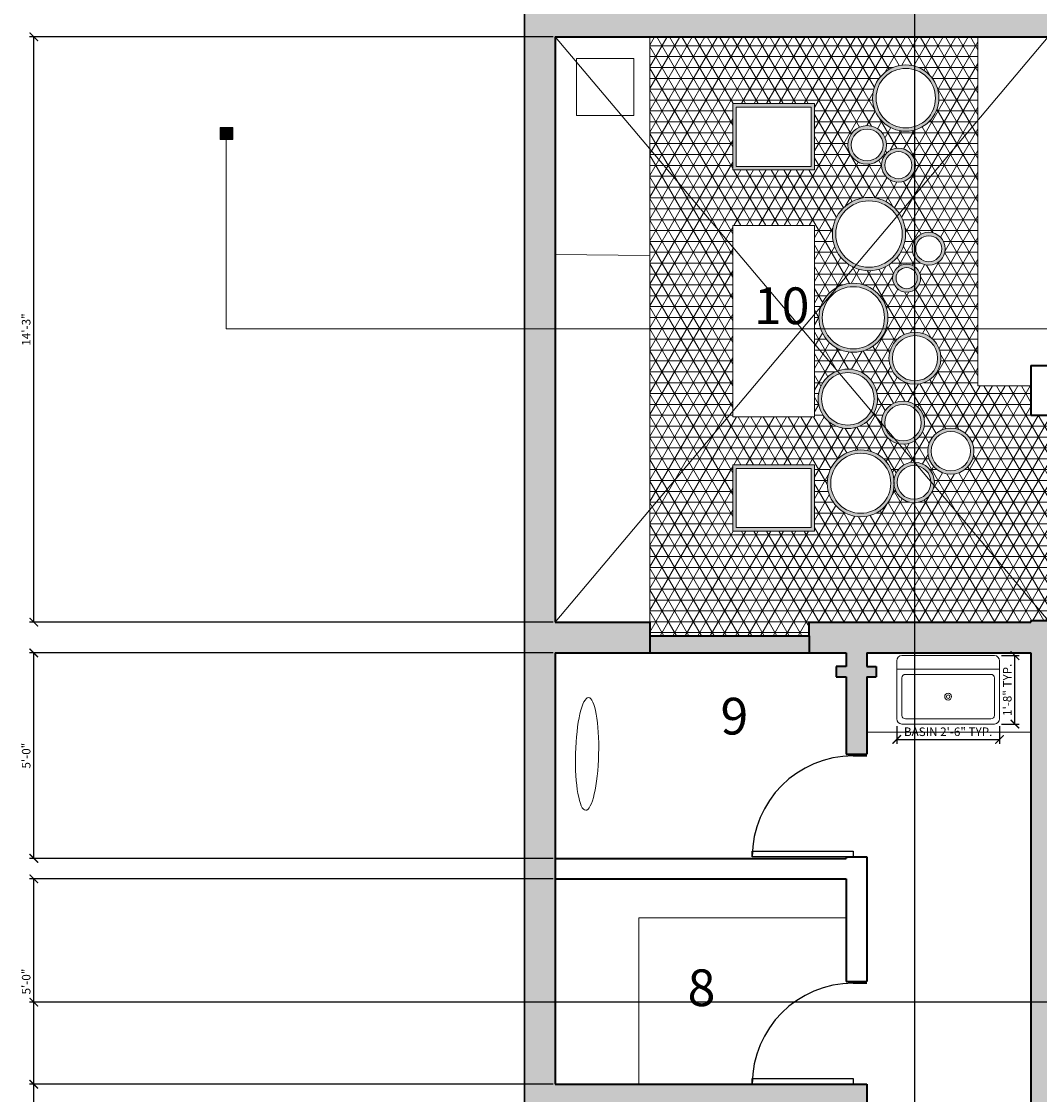
# Model space of a CAD drawing. Units: inches. Extents: x 3122 to 5933, y 1474 to 2995.
# Tile 5 of 12: x 4918 to 5215, y 2326 to 2639. Entities that reach past the tile are written whole.
import ezdxf

# ---------------------------------------------------------------- set-up
doc = ezdxf.new("R2010")
doc.units = ezdxf.units.IN
for name, color, linetype, lineweight in [('A-ANNO-DIMS', 2, 'Continuous', 18), ('A-ANNO-SYMB', 6, 'Continuous', 18), ('A-AREA-IDEN', 7, 'Continuous', 20), ('A-DOOR', 4, 'Continuous', 25), ('A-FLOR-CASE', 8, 'Continuous', 18), ('A-FLOR-FIXT', 9, 'Continuous', 18), ('A-FLOR-OPEN', 8, 'Continuous', 13), ('A-WALL', 7, 'Continuous', 35), ('A-WALL-PATT', 7, 'Continuous', 13), ('C-PROP', 7, 'Continuous', 25), ('L-PLNT', 3, 'Continuous', 18), ('L-PLNT-PATT', 94, 'Continuous', 13)]:
    doc.layers.add(name, color=color, linetype=linetype, lineweight=lineweight)
doc.styles.get("Standard").update_dxf_attribs({"font": 'arial.ttf'})
doc.dimstyles.new('ISO-25', dxfattribs={"dimtxt": 2.5, "dimasz": 2.5, "dimexe": 1.25, "dimexo": 0.625, "dimtad": 1, "dimdec": 0, "dimlunit": 3, "dimtxsty": 'Standard', "dimblk": 'ARCHTICK', "dimcen": 2.5, "dimadec": 0, "dimazin": 0, "dimtfac": 1, "dimtdec": 0, "dimtmove": 0, "dimatfit": 3, "dimfxl": 1, "dimarcsym": 0})

# ---------------------------------------------------------------- blocks, each defined once
blk = doc.blocks.new('*U31')
for p, q in [((0, 0), (0, -100)), ((750, 0), (750, -100))]:
    blk.add_line(p, q)
blk.add_lwpolyline([(0, 0), (0, 750), (43.75, 750), (43.75, 0)], close=True)
blk.add_arc((0, 0), 750, 0, 90)
blk = doc.blocks.new('Sink-single - 30 in top')
blk.add_line((-15, -3.999996), (15, -3.999996))
for points in [[(-13.5, 0), (13.5, 0)], [(-15, -18.499996), (-15, -1.5)], [(15, -1.5), (15, -18.499996)], [(-12.5, -5.499996), (12.5, -5.499996)], [(-13.5, -17.499996), (-13.5, -6.499996)], [(13.5, -6.499996), (13.5, -17.499996)], [(12.5, -18.499996), (-12.5, -18.499996)], [(13.5, -19.999996), (-13.5, -19.999996)]]:
    blk.add_lwpolyline(points)
for radius in [1, 0.5]:
    blk.add_circle((0, -11.999996), radius)
for centre, radius, start, end in [((-13.5, -1.5), 1.5, 90, 180), ((13.5, -1.5), 1.5, 0, 90), ((-12.5, -6.499996), 1, 90, 180), ((12.5, -6.499996), 1, 0, 90), ((-13.5, -18.499996), 1.5, 180, 270), ((-12.5, -17.499996), 1, 180, 270), ((12.5, -17.499996), 1, 270, 0), ((13.5, -18.499996), 1.5, 270, 0)]:
    blk.add_arc(centre, radius, start, end)
blk = doc.blocks.new('SECTION-LINE-END-MARK')
h = blk.add_hatch(color=256)
h.dxf.hatch_style = 1
h.paths.add_polyline_path([(3.68, 3.54), (0, 3.54), (0, 0), (3.68, 0)])
blk.add_lwpolyline([(0, 3.54), (3.68, 3.54), (3.68, 0), (0, 0)], close=True)
blk = doc.blocks.new('_ArchTick')
at = {"color": 0, "linetype": 'ByBlock', "const_width": 0.15}
blk.add_lwpolyline([(-0.5, -0.5), (0.5, 0.5)], dxfattribs=at)
blk = doc.blocks.new('*D58')
at = {"layer": 'A-ANNO-DIMS', "color": 0, "lineweight": -2, "transparency": 16777216}
for p, q in [((5173.76, 2433.31), (5173.76, 2428.18)), ((5203.76, 2433.31), (5203.76, 2428.18)), ((5173.76, 2429.43), (5203.76, 2429.43))]:
    blk.add_line(p, q, dxfattribs=at)
at = {"layer": 'Defpoints', "color": 0, "transparency": 16777216}
for p in [(5173.76, 2433.93), (5203.76, 2433.93), (5203.76, 2429.43)]:
    blk.add_point(p, dxfattribs=at)
at = {"layer": 'A-ANNO-DIMS', "color": 0, "lineweight": -2, "transparency": 16777216, "xscale": 2.5, "yscale": 2.5, "zscale": 2.5, "rotation": 180}
blk.add_blockref('_ArchTick', (5173.76, 2429.43), dxfattribs=at)
at = {"layer": 'A-ANNO-DIMS', "color": 0, "lineweight": -2, "transparency": 16777216, "xscale": 2.5, "yscale": 2.5, "zscale": 2.5}
blk.add_blockref('_ArchTick', (5203.76, 2429.43), dxfattribs=at)
at = {"layer": 'A-ANNO-DIMS', "color": 0, "transparency": 16777216, "insert": (5188.76, 2431.35), "char_height": 2.5, "attachment_point": 5}
blk.add_mtext('BASIN 2\'-6" TYP.', dxfattribs=at)
blk = doc.blocks.new('*D59')
at = {"layer": 'A-ANNO-DIMS', "color": 0, "lineweight": -2, "transparency": 16777216}
for p, q in [((5204.38, 2453.93), (5209.51, 2453.93)), ((5208.26, 2433.93), (5208.26, 2453.93)), ((5204.38, 2433.93), (5209.51, 2433.93))]:
    blk.add_line(p, q, dxfattribs=at)
at = {"layer": 'Defpoints', "color": 0, "transparency": 16777216}
for p in [(5203.76, 2453.93), (5208.26, 2453.93), (5203.76, 2433.93)]:
    blk.add_point(p, dxfattribs=at)
at = {"layer": 'A-ANNO-DIMS', "color": 0, "lineweight": -2, "transparency": 16777216, "xscale": 2.5, "yscale": 2.5, "zscale": 2.5}
for p, rotation in [((5208.26, 2453.93), 90), ((5208.26, 2433.93), 270)]:
    blk.add_blockref('_ArchTick', p, dxfattribs=dict(at, rotation=rotation))
at = {"layer": 'A-ANNO-DIMS', "color": 0, "transparency": 16777216, "insert": (5206.36, 2443.93), "char_height": 2.5, "attachment_point": 5, "rotation": 90}
blk.add_mtext('1\'-8" TYP.', dxfattribs=at)
blk = doc.blocks.new('*D94')
at = {"layer": 'A-ANNO-DIMS', "color": 0, "lineweight": -2, "transparency": 16777216}
for p, q in [((5064.96, 1916.52), (5064.96, 2990.75)), ((5064.96, 2989.5), (5487.87, 2989.5)), ((5487.87, 1916.52), (5487.87, 2990.75))]:
    blk.add_line(p, q, dxfattribs=at)
at = {"layer": 'Defpoints', "color": 0, "transparency": 16777216}
for p in [(5487.87, 2989.5), (5064.96, 1915.9), (5487.87, 1915.9)]:
    blk.add_point(p, dxfattribs=at)
at = {"layer": 'A-ANNO-DIMS', "color": 0, "lineweight": -2, "transparency": 16777216, "xscale": 2.5, "yscale": 2.5, "zscale": 2.5, "rotation": 180}
blk.add_blockref('_ArchTick', (5064.96, 2989.5), dxfattribs=at)
at = {"layer": 'A-ANNO-DIMS', "color": 0, "lineweight": -2, "transparency": 16777216, "xscale": 2.5, "yscale": 2.5, "zscale": 2.5}
blk.add_blockref('_ArchTick', (5487.87, 2989.5), dxfattribs=at)
at = {"layer": 'A-ANNO-DIMS', "color": 0, "transparency": 16777216, "insert": (5276.42, 2991.41), "char_height": 2.5, "attachment_point": 5}
blk.add_mtext('35\'-3"', dxfattribs=at)
blk = doc.blocks.new('*D99')
at = {"layer": 'A-ANNO-DIMS', "color": 0, "lineweight": -2, "transparency": 16777216}
for p, q in [((5073.34, 2388.69), (4920.36, 2388.69)), ((4921.61, 2328.69), (4921.61, 2388.69)), ((5073.34, 2328.69), (4920.36, 2328.69))]:
    blk.add_line(p, q, dxfattribs=at)
at = {"layer": 'Defpoints', "color": 0, "transparency": 16777216}
for p in [(4921.61, 2388.69), (5073.96, 2388.69), (5073.96, 2328.69)]:
    blk.add_point(p, dxfattribs=at)
at = {"layer": 'A-ANNO-DIMS', "color": 0, "lineweight": -2, "transparency": 16777216, "xscale": 2.5, "yscale": 2.5, "zscale": 2.5}
for p, rotation in [((4921.61, 2388.69), 90), ((4921.61, 2328.69), 270)]:
    blk.add_blockref('_ArchTick', p, dxfattribs=dict(at, rotation=rotation))
at = {"layer": 'A-ANNO-DIMS', "color": 0, "transparency": 16777216, "insert": (4919.71, 2358.69), "char_height": 2.5, "attachment_point": 5, "rotation": 90}
blk.add_mtext('5\'-0"', dxfattribs=at)
blk = doc.blocks.new('*D100')
at = {"layer": 'A-ANNO-DIMS', "color": 0, "lineweight": -2, "transparency": 16777216}
for p, q in [((5073.34, 2454.69), (4920.36, 2454.69)), ((4921.61, 2394.69), (4921.61, 2454.69)), ((5073.34, 2394.69), (4920.36, 2394.69))]:
    blk.add_line(p, q, dxfattribs=at)
at = {"layer": 'Defpoints', "color": 0, "transparency": 16777216}
for p in [(4921.61, 2454.69), (5073.96, 2454.69), (5073.96, 2394.69)]:
    blk.add_point(p, dxfattribs=at)
at = {"layer": 'A-ANNO-DIMS', "color": 0, "lineweight": -2, "transparency": 16777216, "xscale": 2.5, "yscale": 2.5, "zscale": 2.5}
for p, rotation in [((4921.61, 2454.69), 90), ((4921.61, 2394.69), 270)]:
    blk.add_blockref('_ArchTick', p, dxfattribs=dict(at, rotation=rotation))
at = {"layer": 'A-ANNO-DIMS', "color": 0, "transparency": 16777216, "insert": (4919.71, 2424.69), "char_height": 2.5, "attachment_point": 5, "rotation": 90}
blk.add_mtext('5\'-0"', dxfattribs=at)
blk = doc.blocks.new('*D101')
at = {"layer": 'A-ANNO-DIMS', "color": 0, "lineweight": -2, "transparency": 16777216}
for p, q in [((5073.34, 2634.69), (4920.36, 2634.69)), ((4921.61, 2463.69), (4921.61, 2634.69)), ((5073.34, 2463.69), (4920.36, 2463.69))]:
    blk.add_line(p, q, dxfattribs=at)
at = {"layer": 'Defpoints', "color": 0, "transparency": 16777216}
for p in [(4921.61, 2634.69), (5073.96, 2634.69), (5073.96, 2463.69)]:
    blk.add_point(p, dxfattribs=at)
at = {"layer": 'A-ANNO-DIMS', "color": 0, "lineweight": -2, "transparency": 16777216, "xscale": 2.5, "yscale": 2.5, "zscale": 2.5}
for p, rotation in [((4921.61, 2634.69), 90), ((4921.61, 2463.69), 270)]:
    blk.add_blockref('_ArchTick', p, dxfattribs=dict(at, rotation=rotation))
at = {"layer": 'A-ANNO-DIMS', "color": 0, "transparency": 16777216, "insert": (4919.71, 2549.19), "char_height": 2.5, "attachment_point": 5, "rotation": 90}
blk.add_mtext('14\'-3"', dxfattribs=at)
blk = doc.blocks.new('*D104')
at = {"layer": 'A-ANNO-DIMS', "color": 0, "lineweight": -2, "transparency": 16777216}
for p, q in [((5427.24, 2352.69), (4920.36, 2352.69)), ((4921.61, 2112.69), (4921.61, 2352.69)), ((5427.24, 2112.69), (4920.36, 2112.69))]:
    blk.add_line(p, q, dxfattribs=at)
at = {"layer": 'Defpoints', "color": 0, "transparency": 16777216}
for p in [(4921.61, 2352.69), (5427.87, 2352.69), (5427.87, 2112.69)]:
    blk.add_point(p, dxfattribs=at)
at = {"layer": 'A-ANNO-DIMS', "color": 0, "lineweight": -2, "transparency": 16777216, "xscale": 2.5, "yscale": 2.5, "zscale": 2.5}
for p, rotation in [((4921.61, 2352.69), 90), ((4921.61, 2112.69), 270)]:
    blk.add_blockref('_ArchTick', p, dxfattribs=dict(at, rotation=rotation))
at = {"layer": 'A-ANNO-DIMS', "color": 0, "transparency": 16777216, "insert": (4919.71, 2232.69), "char_height": 2.5, "attachment_point": 5, "rotation": 90}
blk.add_mtext('20\'-0"', dxfattribs=at)
blk = doc.blocks.new('*D108')
at = {"layer": 'A-ANNO-DIMS', "color": 0, "lineweight": -2, "transparency": 16777216}
for p, q in [((5178.96, 2643.06), (5178.96, 1792.93)), ((5358.96, 2643.06), (5358.96, 1792.93)), ((5178.96, 1794.18), (5358.96, 1794.18))]:
    blk.add_line(p, q, dxfattribs=at)
at = {"layer": 'Defpoints', "color": 0, "transparency": 16777216}
for p in [(5178.96, 2643.69), (5358.96, 2643.69), (5358.96, 1794.18)]:
    blk.add_point(p, dxfattribs=at)
at = {"layer": 'A-ANNO-DIMS', "color": 0, "lineweight": -2, "transparency": 16777216, "xscale": 2.5, "yscale": 2.5, "zscale": 2.5, "rotation": 180}
blk.add_blockref('_ArchTick', (5178.96, 1794.18), dxfattribs=at)
at = {"layer": 'A-ANNO-DIMS', "color": 0, "lineweight": -2, "transparency": 16777216, "xscale": 2.5, "yscale": 2.5, "zscale": 2.5}
blk.add_blockref('_ArchTick', (5358.96, 1794.18), dxfattribs=at)
at = {"layer": 'A-ANNO-DIMS', "color": 0, "transparency": 16777216, "insert": (5268.96, 1796.08), "char_height": 2.5, "attachment_point": 5}
blk.add_mtext('15\'-0"', dxfattribs=at)

msp = doc.modelspace()

# ---------------------------------------------------------------- hatches: boundary and pattern name
at = {"layer": 'A-WALL-PATT'}
h = msp.add_hatch(color=256, dxfattribs=at)
h.dxf.hatch_style = 1
h.paths.add_polyline_path([(5073.96, 2454.69), (5101.59, 2454.69), (5101.59, 2459.69), (5101.59, 2463.69), (5073.96, 2463.69), (5073.96, 2634.69), (5169.96, 2634.69), (5364.96, 2634.69), (5364.96, 2643.69), (5364.96, 2667.06), (5358.96, 2667.06), (5358.96, 2643.69), (5178.96, 2643.69), (5178.96, 2655.69), (5169.96, 2655.69), (5169.96, 2643.69), (5073.96, 2643.69), (5073.96, 2745.9), (5124.13, 2745.9), (5124.13, 2754.9), (5073.96, 2754.9), (5073.96, 2866.9), (5169.96, 2866.9), (5169.96, 2818.9), (5169.96, 2812.9), (5169.96, 2754.9), (5154.13, 2754.9), (5154.13, 2745.9), (5169.96, 2745.9), (5169.96, 2691.69), (5178.96, 2691.69), (5178.96, 2812.9), (5178.96, 2818.9), (5178.96, 2875.9), (5064.96, 2875.9), (5064.96, 2055.71), (5217.96, 2055.71), (5217.96, 2464.19), (5212.96, 2464.19), (5212.96, 2463.69), (5148.19, 2463.69), (5148.19, 2459.69), (5148.19, 2454.69), (5158.96, 2454.69), (5158.96, 2450.72), (5156.04, 2450.72), (5156.04, 2447.72), (5158.96, 2447.72), (5158.96, 2425.1), (5164.96, 2425.1), (5164.96, 2447.72), (5167.71, 2447.72), (5167.71, 2450.72), (5164.96, 2450.72), (5164.96, 2454.69), (5212.96, 2454.69), (5212.96, 2064.71), (5073.96, 2064.71), (5073.96, 2322.69), (5158.96, 2322.69), (5164.96, 2322.69), (5164.96, 2328.69), (5158.96, 2328.69), (5073.96, 2328.69)])
h = msp.add_hatch(color=256, dxfattribs=at)
h.dxf.hatch_style = 1
h.paths.add_polyline_path([(5148.19, 2459.69), (5101.59, 2459.69), (5101.59, 2454.69), (5148.19, 2454.69)])
at = {"layer": 'L-PLNT-PATT'}
h = msp.add_hatch(dxfattribs=at)
h.set_pattern_fill('NET3', color=256)
h.paths.add_polyline_path([(5217.96, 2524.19), (5212.96, 2524.19), (5212.96, 2532.69), (5197.46, 2532.69), (5197.46, 2634.69), (5169.96, 2634.69), (5101.59, 2634.69), (5101.59, 2463.69), (5101.59, 2459.69), (5148.19, 2459.69), (5148.19, 2463.69), (5212.96, 2463.69), (5212.96, 2464.19), (5217.96, 2464.19)])
h.paths.add_polyline_path([(5125.86, 2509.63), (5149.73, 2509.63), (5149.73, 2490.31), (5125.86, 2490.31)], flags=16)
h.paths.add_polyline_path([(5125.86, 2523.69), (5125.86, 2579.54), (5149.73, 2579.54), (5149.73, 2523.69)], flags=16)
h.paths.add_polyline_path([(5172.93, 2505.39, -0.929737), (5184.73, 2504.53, -0.91381), (5172.96, 2503.47, -0.960136), (5153.44, 2504.26, -0.943722)], flags=16)
h.paths.add_polyline_path([(5150.78, 2528.95, -1), (5168.14, 2528.95, -1)], flags=16)
h.paths.add_polyline_path([(5150.99, 2552.62, -1), (5171.14, 2552.62, -1)], flags=16)
h.paths.add_polyline_path([(5169.25, 2521.97, -1), (5181.9, 2521.97, -1)], flags=16)
h.paths.add_polyline_path([(5171.47, 2540.81, -1), (5186.66, 2540.81, -1)], flags=16)
h.paths.add_polyline_path([(5182.81, 2513.65, -1), (5196.27, 2513.65, -1)], flags=16)
h.paths.add_polyline_path([(5154.93, 2577.08, -1), (5176.33, 2577.08, -1)], flags=16)
h.paths.add_polyline_path([(5172.55, 2564.2, -1), (5180.74, 2564.2, -1)], flags=16)
h.paths.add_polyline_path([(5178.29, 2572.78, -1), (5187.9, 2572.78, -1)], flags=16)
h.paths.add_polyline_path([(5125.86, 2595.84), (5125.86, 2615.17), (5149.73, 2615.17), (5149.73, 2595.84)], flags=16)
h.paths.add_polyline_path([(5169.27, 2597.2, -1), (5179.18, 2597.2, -1)], flags=16)
h.paths.add_polyline_path([(5159.45, 2603.11, -1), (5170.74, 2603.11, -1)], flags=16)
h.paths.add_polyline_path([(5166.7, 2616.79, -1), (5186.05, 2616.79, -1)], flags=16)
h.paths.add_polyline_path([(5129.27, 2547.83), (5151.41, 2547.84), (5151.4, 2564.27), (5129.26, 2564.26)], flags=24)
h = msp.add_hatch(color=256, dxfattribs=at)
h.dxf.hatch_style = 1
h.paths.add_polyline_path([(5149.73, 2509.63), (5125.86, 2509.63), (5125.86, 2490.31), (5149.73, 2490.31)])
h.paths.add_polyline_path([(5148.73, 2491.31), (5126.86, 2491.31), (5126.86, 2508.63), (5148.73, 2508.63)], flags=16)
h.paths.add_polyline_path([(5153.44, 2504.26, 1), (5172.99, 2504.26, 1)])
h.paths.add_polyline_path([(5171.99, 2504.26, -1), (5154.44, 2504.26, -1)], flags=16)
h.paths.add_polyline_path([(5184.73, 2504.53, 0.929737), (5172.93, 2505.39, -0.028954), (5172.99, 2504.26, -0.020337), (5172.96, 2503.47, 0.91381)])
h.paths.add_polyline_path([(5173.86, 2504.53, -1), (5183.73, 2504.53, -1)], flags=16)
h.paths.add_polyline_path([(5196.27, 2513.65, 1), (5182.81, 2513.65, 1)])
h.paths.add_polyline_path([(5183.81, 2513.65, -1), (5195.27, 2513.65, -1)], flags=16)
h.paths.add_polyline_path([(5181.9, 2521.97, 1), (5169.25, 2521.97, 1)])
h.paths.add_polyline_path([(5170.25, 2521.97, -1), (5180.9, 2521.97, -1)], flags=16)
h.paths.add_polyline_path([(5168.14, 2528.95, 1), (5150.78, 2528.95, 1)])
h.paths.add_polyline_path([(5151.78, 2528.95, -1), (5167.14, 2528.95, -1)], flags=16)
h.paths.add_polyline_path([(5186.66, 2540.81, 1), (5171.47, 2540.81, 1)])
h.paths.add_polyline_path([(5172.47, 2540.81, -1), (5185.66, 2540.81, -1)], flags=16)
h.paths.add_polyline_path([(5170.14, 2552.62, 1), (5151.99, 2552.62, 1)], flags=0)
h.paths.add_polyline_path([(5171.14, 2552.62, 1), (5150.99, 2552.62, 1)])
h.paths.add_polyline_path([(5151.99, 2552.62, -1), (5170.14, 2552.62, -1)], flags=16)
h.paths.add_polyline_path([(5180.74, 2564.2, 1), (5172.55, 2564.2, 1)])
h.paths.add_polyline_path([(5173.55, 2564.2, -1), (5179.74, 2564.2, -1)], flags=16)
h.paths.add_polyline_path([(5187.9, 2572.78, 1), (5178.29, 2572.78, 1)])
h.paths.add_polyline_path([(5179.29, 2572.78, -1), (5186.9, 2572.78, -1)], flags=16)
h.paths.add_polyline_path([(5176.33, 2577.08, 1), (5154.93, 2577.08, 1)])
h.paths.add_polyline_path([(5155.93, 2577.08, -1), (5175.33, 2577.08, -1)], flags=16)
h.paths.add_polyline_path([(5149.73, 2615.17), (5125.86, 2615.17), (5125.86, 2595.84), (5149.73, 2595.84)])
h.paths.add_polyline_path([(5126.86, 2596.84), (5126.86, 2614.17), (5148.73, 2614.17), (5148.73, 2596.84)], flags=16)
h.paths.add_polyline_path([(5170.74, 2603.11, 1), (5159.45, 2603.11, 1)])
h.paths.add_polyline_path([(5160.45, 2603.11, -1), (5169.74, 2603.11, -1)], flags=16)
h.paths.add_polyline_path([(5179.18, 2597.2, 1), (5169.27, 2597.2, 1)])
h.paths.add_polyline_path([(5170.27, 2597.2, -1), (5178.18, 2597.2, -1)], flags=16)
h.paths.add_polyline_path([(5166.7, 2616.79, 1), (5186.05, 2616.79, 1)])
h.paths.add_polyline_path([(5185.05, 2616.79, -1), (5167.7, 2616.79, -1)], flags=16)

# ---------------------------------------------------------------- linework, layer by layer
at = {"layer": 'A-ANNO-SYMB'}
for p, q in [((4977.78, 2549.4), (4977.78, 2604.65)), ((4977.78, 2604.65), (4977.78, 2549.4)), ((5874.48, 2549.4), (4977.78, 2549.4))]:
    msp.add_line(p, q, dxfattribs=at)
at = {"layer": 'A-FLOR-CASE'}
for p, q in [((5158.96, 2377.27), (5098.38, 2377.27)), ((5098.38, 2377.27), (5098.38, 2328.69))]:
    msp.add_line(p, q, dxfattribs=at)
at = {"layer": 'A-FLOR-FIXT'}
msp.add_line((5212.96, 2431.54), (5164.96, 2431.54), dxfattribs=at)
msp.add_ellipse((5083.27, 2425.19), major_axis=(-0.41, -16.46), ratio=0.204663, dxfattribs=at)
at = {"layer": 'A-FLOR-OPEN'}
for p, q in [((5073.96, 2634.69), (5217.96, 2464.19)), ((5073.96, 2463.69), (5217.96, 2634.69))]:
    msp.add_line(p, q, dxfattribs=at)
at = {"layer": 'A-WALL'}
for p, q in [((5073.96, 2634.69), (5169.96, 2634.69)), ((5073.96, 2634.69), (5073.96, 2463.69)), ((5169.96, 2634.69), (5364.96, 2634.69)), ((5212.96, 2538.69), (5358.96, 2538.69)), ((5212.96, 2538.69), (5212.96, 2524.19)), ((5212.96, 2524.19), (5217.96, 2524.19)), ((5212.96, 2464.19), (5217.96, 2464.19)), ((5212.96, 2464.19), (5212.96, 2463.69)), ((5073.96, 2463.69), (5101.59, 2463.69)), ((5073.96, 2463.69), (5101.59, 2463.69)), ((5101.59, 2463.69), (5101.59, 2459.69)), ((5148.19, 2459.69), (5148.19, 2463.69)), ((5148.19, 2463.69), (5212.96, 2463.69)), ((5101.59, 2459.69), (5148.19, 2459.69)), ((5101.59, 2459.69), (5101.59, 2454.69)), ((5148.19, 2459.69), (5148.19, 2454.69)), ((5073.96, 2454.69), (5158.96, 2454.69)), ((5073.96, 2454.69), (5073.96, 2328.69)), ((5158.96, 2454.69), (5158.96, 2450.72)), ((5164.96, 2454.69), (5164.96, 2450.72)), ((5164.96, 2454.69), (5212.96, 2454.69)), ((5212.96, 2454.69), (5212.96, 2064.71)), ((5158.96, 2450.72), (5156.04, 2450.72)), ((5156.04, 2450.72), (5156.04, 2447.72)), ((5164.96, 2450.72), (5167.71, 2450.72)), ((5167.71, 2450.72), (5167.71, 2447.72)), ((5156.04, 2447.72), (5158.96, 2447.72)), ((5158.96, 2447.72), (5158.96, 2425.1)), ((5164.96, 2447.72), (5167.71, 2447.72)), ((5164.96, 2447.72), (5164.96, 2425.1)), ((5158.96, 2425.1), (5164.96, 2425.1)), ((5073.96, 2394.69), (5158.96, 2394.69)), ((5158.96, 2395.1), (5164.96, 2395.1)), ((5158.96, 2395.1), (5158.96, 2394.69)), ((5164.96, 2395.1), (5164.96, 2358.69)), ((5073.96, 2388.69), (5158.96, 2388.69)), ((5158.96, 2388.69), (5158.96, 2358.69)), ((5158.96, 2358.69), (5164.96, 2358.69)), ((5073.96, 2328.69), (5158.96, 2328.69)), ((5158.96, 2328.69), (5164.96, 2328.69)), ((5164.96, 2328.69), (5164.96, 2322.69))]:
    msp.add_line(p, q, dxfattribs=at)
at = {"layer": 'C-PROP'}
msp.add_line((5064.96, 2875.9), (5064.96, 1915.9), dxfattribs=at)
at = {"layer": 'L-PLNT'}
for p, q in [((5101.59, 2634.69), (5101.59, 2463.69)), ((5197.46, 2634.69), (5197.46, 2532.69)), ((5101.59, 2570.78), (5073.96, 2571.11)), ((5197.46, 2532.69), (5212.96, 2532.69))]:
    msp.add_line(p, q, dxfattribs=at)
for points in [[(5080.22, 2628.4), (5096.91, 2628.4), (5096.91, 2611.73), (5080.22, 2611.73)], [(5125.86, 2615.17), (5149.73, 2615.17), (5149.73, 2595.84), (5125.86, 2595.84)], [(5126.86, 2614.17), (5148.73, 2614.17), (5148.73, 2596.84), (5126.86, 2596.84)], [(5125.86, 2579.54), (5149.73, 2579.54), (5149.73, 2523.69), (5125.86, 2523.69)], [(5125.86, 2509.63), (5149.73, 2509.63), (5149.73, 2490.31), (5125.86, 2490.31)], [(5126.86, 2508.63), (5148.73, 2508.63), (5148.73, 2491.31), (5126.86, 2491.31)]]:
    msp.add_lwpolyline(points, close=True, dxfattribs=at)
for centre, radius in [((5176.38, 2616.79), 9.68), ((5176.38, 2616.79), 8.68), ((5165.09, 2603.11), 5.64), ((5165.09, 2603.11), 4.64), ((5174.23, 2597.2), 4.95), ((5174.23, 2597.2), 3.95), ((5165.63, 2577.08), 10.7), ((5165.63, 2577.08), 9.7), ((5183.09, 2572.78), 4.8), ((5183.09, 2572.78), 3.8), ((5176.64, 2564.2), 4.09), ((5176.64, 2564.2), 3.09), ((5161.07, 2552.62), 10.08), ((5161.07, 2552.62), 9.08), ((5179.07, 2540.81), 7.6), ((5179.07, 2540.81), 6.6), ((5159.46, 2528.95), 8.68), ((5159.46, 2528.95), 7.68), ((5175.58, 2521.97), 6.32), ((5175.58, 2521.97), 5.32), ((5189.54, 2513.65), 6.73), ((5189.54, 2513.65), 5.73), ((5163.22, 2504.26), 9.77), ((5163.22, 2504.26), 8.77), ((5178.8, 2504.53), 5.93), ((5178.8, 2504.53), 4.93)]:
    msp.add_circle(centre, radius, dxfattribs=at)

# ---------------------------------------------------------------- block references
at = {"layer": 'A-ANNO-SYMB'}
msp.add_blockref('SECTION-LINE-END-MARK', (4976.11, 2604.67), dxfattribs=at)
at = {"layer": 'A-DOOR', "xscale": 0.0393700787401575, "yscale": 0.0393700787401575, "zscale": 0.0393700787401575, "rotation": 90}
for p in [(5161.03, 2395.1), (5161.03, 2328.69)]:
    msp.add_blockref('*U31', p, dxfattribs=at)
at = {"layer": 'A-FLOR-FIXT'}
msp.add_blockref('Sink-single - 30 in top', (5188.76, 2453.93), dxfattribs=at)

# ---------------------------------------------------------------- texts
at = {"layer": 'A-AREA-IDEN'}
for s, height, p in [('10', 10.725, (5132, 2550.75)), ('9', 10.72, (5122.25, 2430.87)), ('8', 10.72, (5112.63, 2351.53))]:
    msp.add_text(s, height=height, rotation=0.0333, dxfattribs=at).set_placement(p)

# ---------------------------------------------------------------- dimensions: what is measured, and where the dimension line sits
at = {"layer": 'A-ANNO-DIMS'}
for base, p1, p2, picture, middle in [((5487.87, 2989.5), (5064.96, 1915.9), (5487.87, 1915.9), '*D94', (5276.42, 2991.41)), ((5358.96, 1794.18), (5178.96, 2643.69), (5358.96, 2643.69), '*D108', (5268.96, 1796.08))]:
    dim = msp.add_linear_dim(base=base, p1=p1, p2=p2, dimstyle='ISO-25', override={"dimdec": 1, "dimlfac": 1, "dimrnd": 0, "dimzin": 1, "dimdsep": 46, "dimlunit": 4, "dimfrac": 2}, dxfattribs=at)
    dim.commit()
    dim.dimension.update_dxf_attribs({"geometry": picture, "text_midpoint": middle})
for base, p1, p2, picture, middle in [((4921.61, 2634.69), (5073.96, 2463.69), (5073.96, 2634.69), '*D101', (4919.71, 2549.19)), ((4921.61, 2454.69), (5073.96, 2394.69), (5073.96, 2454.69), '*D100', (4919.71, 2424.69)), ((4921.61, 2388.69), (5073.96, 2328.69), (5073.96, 2388.69), '*D99', (4919.71, 2358.69)), ((4921.61, 2352.69), (5427.87, 2112.69), (5427.87, 2352.69), '*D104', (4919.71, 2232.69))]:
    dim = msp.add_linear_dim(base=base, p1=p1, p2=p2, angle=90, dimstyle='ISO-25', override={"dimdec": 1, "dimlfac": 1, "dimrnd": 0, "dimzin": 1, "dimdsep": 46, "dimlunit": 4, "dimfrac": 2}, dxfattribs=at)
    dim.commit()
    dim.dimension.update_dxf_attribs({"geometry": picture, "text_midpoint": middle})
dim = msp.add_linear_dim(base=(5208.26, 2453.93), p1=(5203.76, 2433.93), p2=(5203.76, 2453.93), angle=90, text='<> TYP.', dimstyle='ISO-25', override={"dimdec": 1, "dimlfac": 1, "dimrnd": 0, "dimzin": 1, "dimdsep": 46, "dimlunit": 4, "dimfrac": 2}, dxfattribs=at)
dim.commit()
dim.dimension.update_dxf_attribs({"geometry": '*D59', "text_midpoint": (5206.36, 2443.93)})
dim = msp.add_linear_dim(base=(5203.76, 2429.43), p1=(5173.76, 2433.93), p2=(5203.76, 2433.93), text='BASIN <> TYP.', dimstyle='ISO-25', override={"dimdec": 1, "dimlfac": 1, "dimrnd": 0, "dimzin": 1, "dimdsep": 46, "dimlunit": 4, "dimfrac": 2}, dxfattribs=at)
dim.commit()
dim.dimension.update_dxf_attribs({"geometry": '*D58', "text_midpoint": (5188.76, 2431.35)})

doc.saveas('drawing.dxf')
